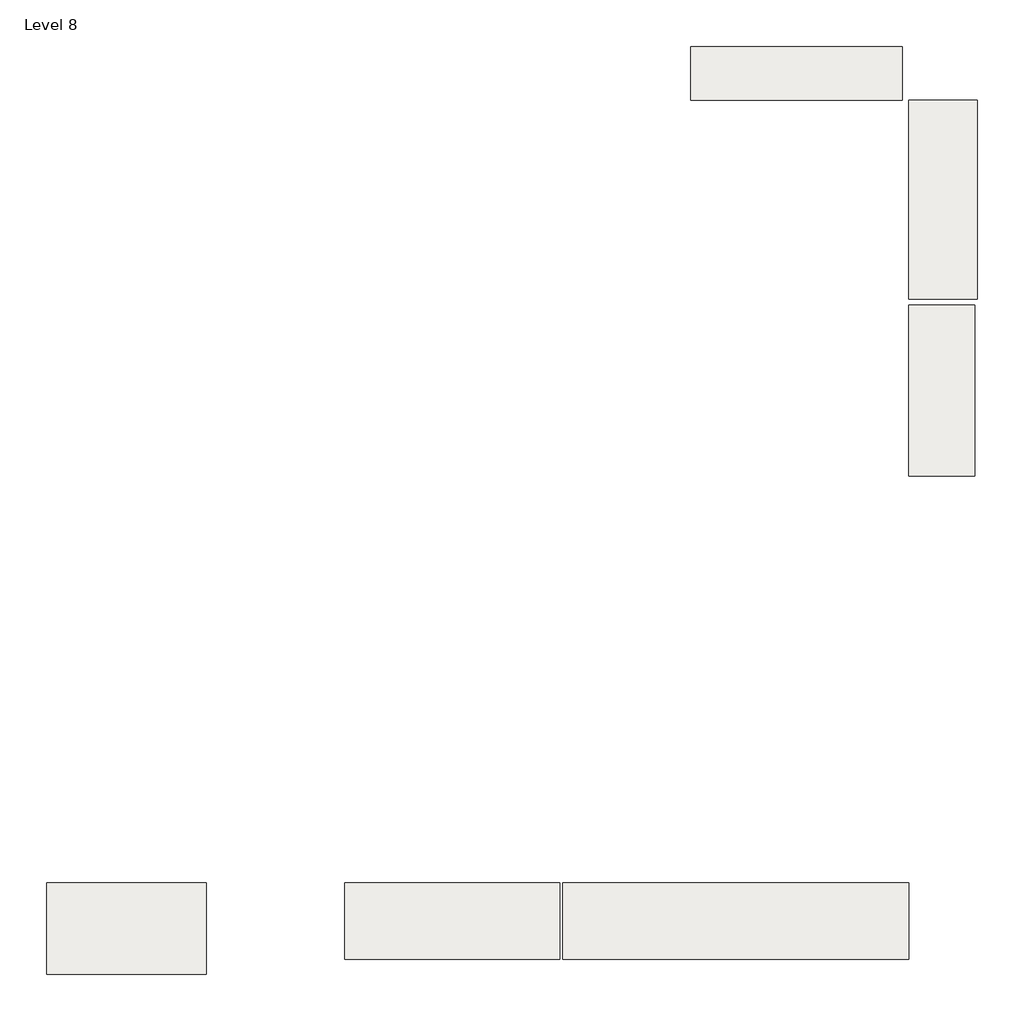
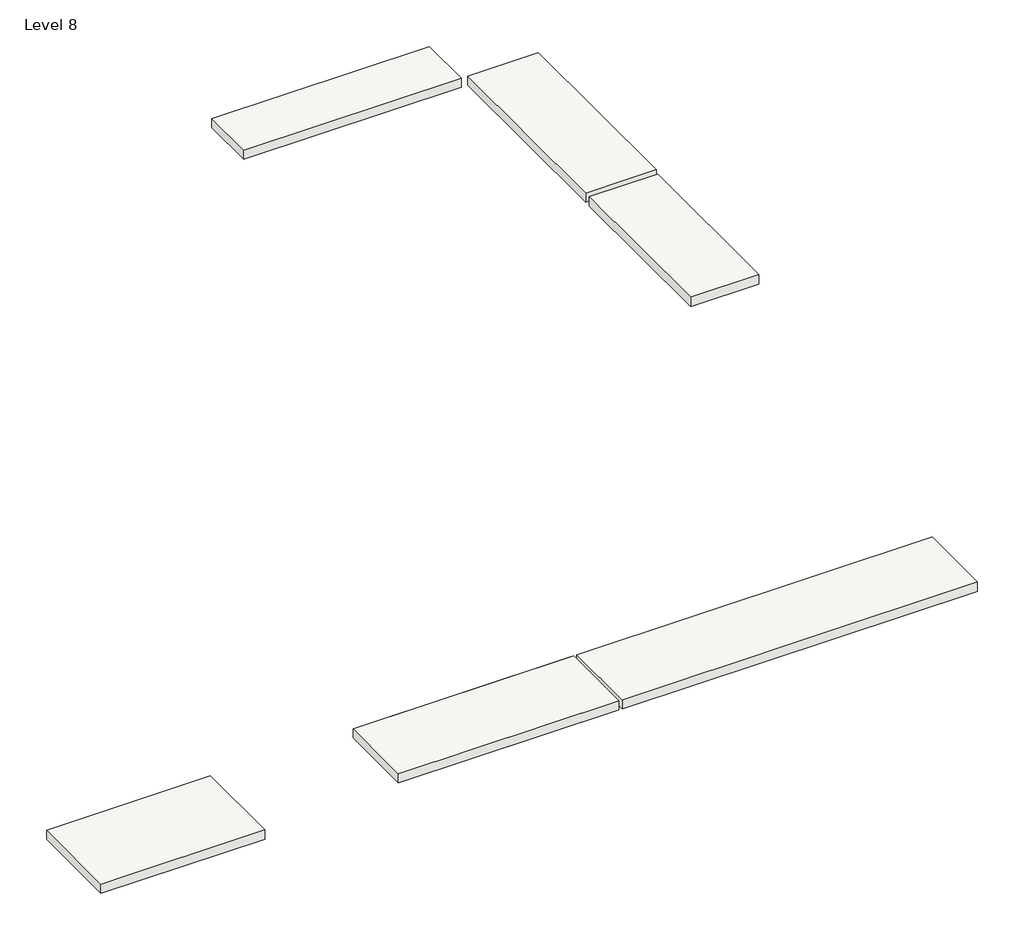
# One storey: 8 slabs.
"""IFC4 building model written with IfcOpenShell, lengths in millimetres."""

from ifc_helpers import new_model, si_unit, frame, origin, place, context, project, spatial, polyline, outline, extrude, element, save

model = new_model("IFC4")

# Units and contexts
model_context = context("Model", 3, world=origin())
ifc_project = project(units=[si_unit("LENGTHUNIT", "METRE", prefix="MILLI")], contexts=[model_context])

# Site, building, storey
site = spatial("IfcSite", under=ifc_project)
building = spatial("IfcBuilding", under=site)
storey = spatial("IfcBuildingStorey", under=building, Name="Level 8", Elevation=6400.8)

# Slabs
placement = place(None, origin())
element("IfcSlab", 1, at=placement, inside=storey, context=model_context, shape_type="SweptSolid", body=[
    extrude(outline(polyline([(14106.5361222, -10428.1762475), (14106.5361222, -12886.3749501), (2981.3361222, -12886.3749501), (2981.3361222, -10428.1762475), (14106.5361222, -10428.1762475)])), frame((0.0, 0.0, 6096.0), z_axis=(0.0, 0.0, 1.0), x_axis=(1.0, 0.0, 0.0)), (0.0, 0.0, 1.0), 304.8),
])
element("IfcSlab", 2, at=placement, inside=storey, context=model_context, shape_type="SweptSolid", body=[
    extrude(outline(polyline([(-8499.4638778, -10428.1762475), (-8499.4638778, -13374.5762475), (-13630.2638778, -13374.5762475), (-13630.2638778, -10428.1762475), (-8499.4638778, -10428.1762475)])), frame((0.0, 0.0, 6096.0), z_axis=(0.0, 0.0, 1.0), x_axis=(1.0, 0.0, 0.0)), (0.0, 0.0, 1.0), 304.8),
])
element("IfcSlab", 3, at=placement, inside=storey, context=model_context, shape_type="SweptSolid", body=[
    extrude(outline(polyline([(2778.1361222, -10428.1762475), (2778.1361222, -12886.3749501), (-4029.0638778, -12886.3749501), (-4029.0638778, -10428.1762475), (2778.1361222, -10428.1762475)])), frame((0.0, 0.0, 6096.0), z_axis=(0.0, 0.0, 1.0), x_axis=(1.0, 0.0, 0.0)), (0.0, 0.0, 1.0), 304.8),
])
element("IfcSlab", 4, at=placement, inside=storey, context=model_context, shape_type="SweptSolid", body=[
    extrude(outline(polyline([(16240.1361222, 8164.6237525), (16240.1361222, 2678.2237525), (14106.5361222, 2678.2237525), (14106.5361222, 8164.6237525), (16240.1361222, 8164.6237525)])), frame((0.0, 0.0, 6096.0), z_axis=(0.0, 0.0, 1.0), x_axis=(1.0, 0.0, 0.0)), (0.0, 0.0, 1.0), 304.8),
])
element("IfcSlab", 5, at=placement, inside=storey, context=model_context, shape_type="SweptSolid", body=[
    extrude(outline(polyline([(16321.4289933, 14768.6237525), (16321.4289933, 8367.8237525), (14106.5361222, 8367.8237525), (14106.5361222, 14768.6237525), (16321.4289933, 14768.6237525)])), frame((0.0, 0.0, 6096.0), z_axis=(0.0, 0.0, 1.0), x_axis=(1.0, 0.0, 0.0)), (0.0, 0.0, 1.0), 304.8),
])
element("IfcSlab", 6, ObjectType="Generic - 12\"", at=placement, inside=storey, context=model_context, shape_type="SweptSolid", body=[
    extrude(outline(polyline([(2879.7361222, -10428.1762475), (2879.7361222, -12886.3749501), (-4029.0638778, -12886.3749501), (-4029.0638778, -10428.1762475), (2879.7361222, -10428.1762475)])), frame((0.0, 0.0, 6096.0), z_axis=(0.0, 0.0, 1.0), x_axis=(1.0, 0.0, 0.0)), (0.0, 0.0, 1.0), 304.8),
])
element("IfcSlab", 7, ObjectType="Generic - 12\"", at=placement, inside=storey, context=model_context, shape_type="SweptSolid", body=[
    extrude(outline(polyline([(16240.1361222, 2678.2237525), (14106.5361222, 2678.2237525), (14106.5361222, 8164.6237525), (16240.1361222, 8164.6237525), (16240.1361222, 2678.2237525)])), frame((0.0, 0.0, 6096.0), z_axis=(0.0, 0.0, 1.0), x_axis=(1.0, 0.0, 0.0)), (0.0, 0.0, 1.0), 304.8),
])
element("IfcSlab", 8, ObjectType="Generic - 12\"", at=placement, inside=storey, context=model_context, shape_type="SweptSolid", body=[
    extrude(outline(polyline([(13903.3361222, 14768.6237525), (7096.1361222, 14768.6237525), (7096.1361222, 16495.8237525), (13903.3361222, 16495.8237525), (13903.3361222, 14768.6237525)])), frame((0.0, 0.0, 6096.0), z_axis=(0.0, 0.0, 1.0), x_axis=(1.0, 0.0, 0.0)), (0.0, 0.0, 1.0), 304.8),
])

save(model, "model.ifc")

# Revit data of these elements
# Type
#   Assembly Code = "B1010"
#   Function = 0
#   Layers, outside or top first: 1' - 0" "Tile, Porcelain, 4in" (function 1)
# Type "Generic - 12\""
#   Assembly Code = "B1010"
#   Function = 0
#   Layers, outside or top first: 1' - 0" no material (function 1)
# Elements 1, 2, 3, 4, 5 (IfcSlab)
#   Height Offset From Level = 0' - 0"
#   Phase Created = New Construction
#   Materials on its faces: "Tile, Porcelain, 4in"
# Elements 6, 7, 8 (IfcSlab, "Generic - 12\"")
#   Height Offset From Level = 0' - 0"
#   Phase Created = New Construction
#   Materials on its faces: "Default Floor"
# Materials
#   "Tile, Porcelain, 4in": class "Generic", colour RGB 89 87 158, transparency 0, Description = "Porcelain tile, 4\", white", Cost = 0
#   "Default Floor": colour RGB 128 128 128, transparency 0
